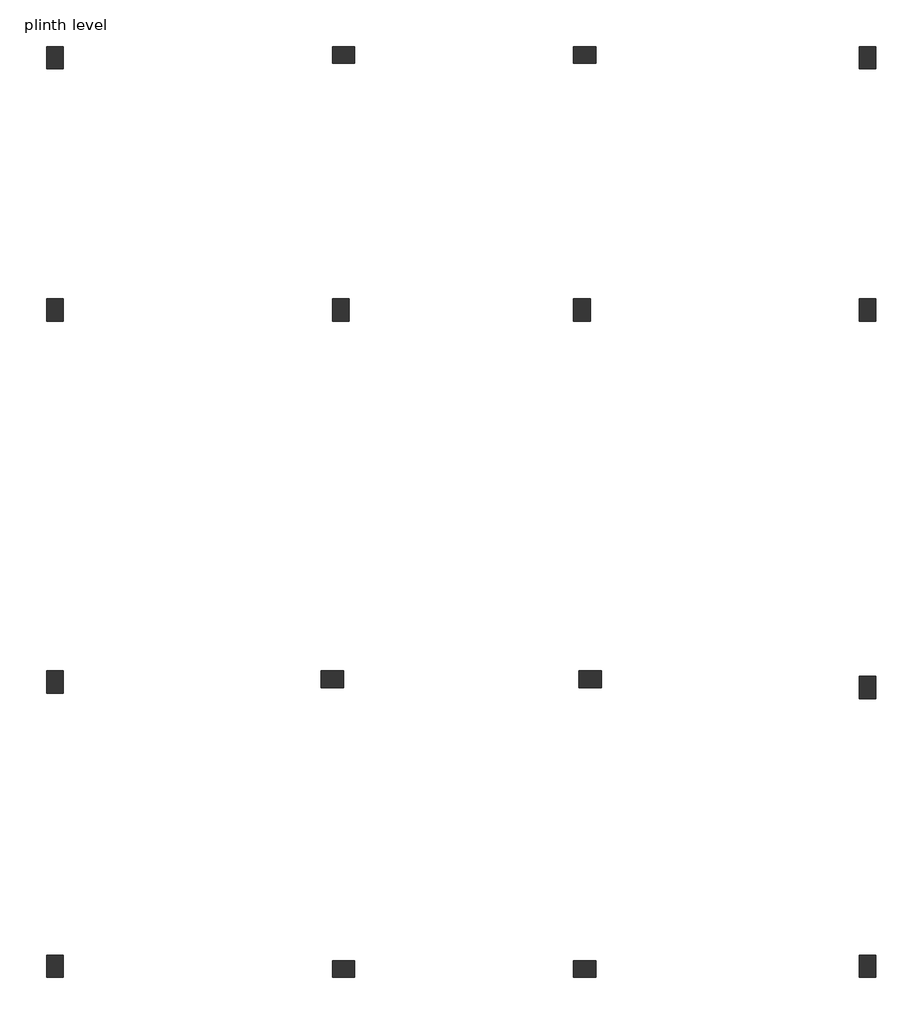
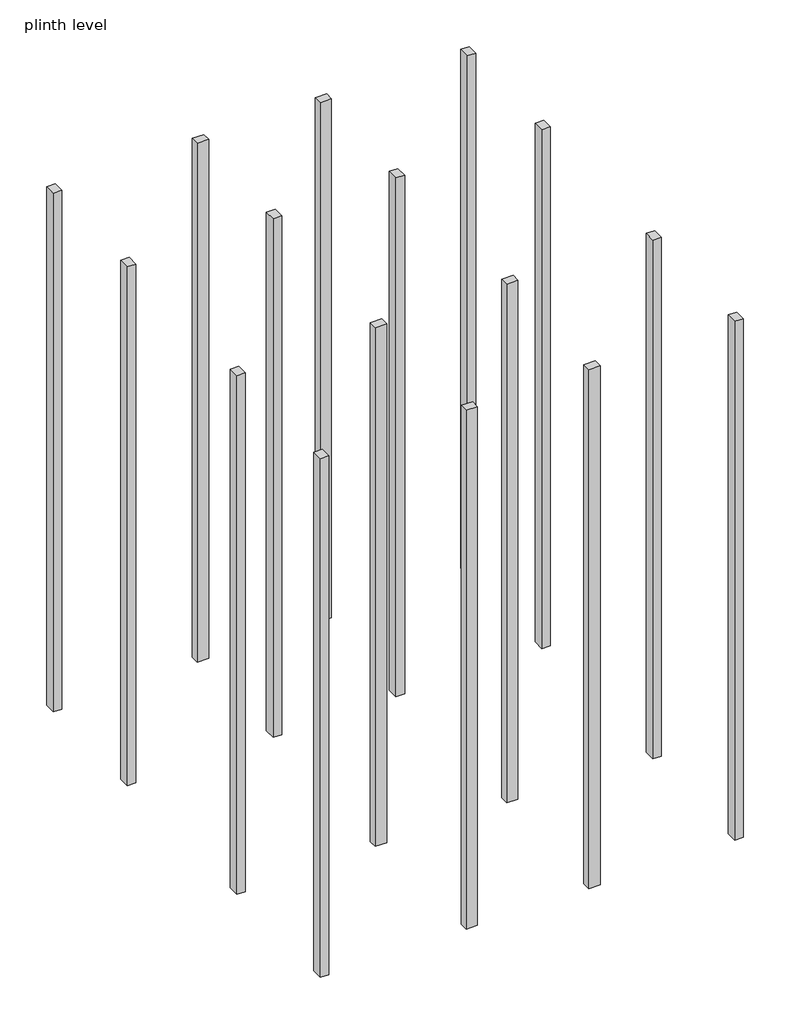
# One storey: 16 columns.
"""IFC4 building model written with IfcOpenShell, lengths in millimetres."""

from ifc_helpers import new_model, si_unit, origin, place, context, project, spatial, faceted_brep, element, save

model = new_model("IFC4")

# Units and contexts
model_context = context("Model", 3, world=origin())
ifc_project = project(units=[si_unit("LENGTHUNIT", "METRE", prefix="MILLI")], contexts=[model_context])

# Site, building, storey
site = spatial("IfcSite", under=ifc_project)
building = spatial("IfcBuilding", under=site)
storey = spatial("IfcBuildingStorey", under=building, Name="plinth level", Elevation=-1219.2)

# Columns
placement = place(None, origin())
element("IfcColumn", 1, ObjectType="Concrete-Rectangular-Column", at=placement, inside=storey, context=model_context, shape_type="Brep", body=[
    faceted_brep([(-12413.6124084, 10180.7961804, -1219.2), (-12413.6124084, 9875.9961804, -1219.2), (-12642.2124084, 9875.9961804, -1219.2), (-12642.2124084, 10180.7961804, -1219.2), (-12413.6124084, 10180.7961804, 13411.2), (-12413.6124084, 9875.9961804, 13411.2), (-12413.6124084, 9875.9961804, 609.6), (-12413.6124084, 9875.9961804, 304.8), (-12642.2124084, 9875.9961804, 13411.2), (-12642.2124084, 9875.9961804, 609.6), (-12642.2124084, 9875.9961804, 304.8), (-12642.2124084, 10180.7961804, 13411.2)], [[[0, 1, 2, 3]], [[4, 5, 6, 7, 1, 0]], [[5, 8, 9, 10, 2, 1, 7, 6]], [[8, 11, 3, 2, 10, 9]], [[11, 4, 0, 3]], [[4, 11, 8, 5]]]),
])
element("IfcColumn", 2, ObjectType="Concrete-Rectangular-Column", at=placement, inside=storey, context=model_context, shape_type="Brep", body=[
    faceted_brep([(-8756.0124084, 10180.7961804, -1219.2), (-8451.2124084, 10180.7961804, -1219.2), (-8451.2124084, 9952.1961804, -1219.2), (-8756.0124084, 9952.1961804, -1219.2), (-8756.0124084, 10180.7961804, 13411.2), (-8451.2124084, 10180.7961804, 13411.2), (-8451.2124084, 9952.1961804, 13411.2), (-8451.2124084, 9952.1961804, 10210.8), (-8451.2124084, 9952.1961804, 9906.0), (-8451.2124084, 9952.1961804, 7010.4), (-8451.2124084, 9952.1961804, 6705.6), (-8451.2124084, 9952.1961804, 3810.0), (-8451.2124084, 9952.1961804, 3505.2), (-8451.2124084, 9952.1961804, 609.6), (-8451.2124084, 9952.1961804, 304.8), (-8756.0124084, 9952.1961804, 13411.2), (-8756.0124084, 9952.1961804, 10210.8), (-8756.0124084, 9952.1961804, 9906.0), (-8756.0124084, 9952.1961804, 7010.4), (-8756.0124084, 9952.1961804, 6705.6), (-8756.0124084, 9952.1961804, 3810.0), (-8756.0124084, 9952.1961804, 3505.2), (-8756.0124084, 9952.1961804, 609.6), (-8756.0124084, 9952.1961804, 304.8)], [[[0, 1, 2, 3]], [[4, 5, 1, 0]], [[5, 6, 7, 8, 9, 10, 11, 12, 13, 14, 2, 1]], [[6, 15, 16, 17, 18, 19, 20, 21, 22, 23, 3, 2, 14, 13, 12, 11, 10, 9, 8, 7]], [[15, 4, 0, 3, 23, 22, 21, 20, 19, 18, 17, 16]], [[4, 15, 6, 5]]]),
])
element("IfcColumn", 3, ObjectType="Concrete-Rectangular-Column", at=placement, inside=storey, context=model_context, shape_type="Brep", body=[
    faceted_brep([(-5479.4124084, 10180.7961804, -1219.2), (-5174.6124084, 10180.7961804, -1219.2), (-5174.6124084, 9952.1961804, -1219.2), (-5479.4124084, 9952.1961804, -1219.2), (-5479.4124084, 10180.7961804, 13411.2), (-5174.6124084, 10180.7961804, 13411.2), (-5174.6124084, 9952.1961804, 13411.2), (-5174.6124084, 9952.1961804, 10210.8), (-5174.6124084, 9952.1961804, 9906.0), (-5174.6124084, 9952.1961804, 7010.4), (-5174.6124084, 9952.1961804, 6705.6), (-5174.6124084, 9952.1961804, 3810.0), (-5174.6124084, 9952.1961804, 3505.2), (-5174.6124084, 9952.1961804, 609.6), (-5174.6124084, 9952.1961804, 304.8), (-5479.4124084, 9952.1961804, 13411.2), (-5479.4124084, 9952.1961804, 10210.8), (-5479.4124084, 9952.1961804, 9906.0), (-5479.4124084, 9952.1961804, 7010.4), (-5479.4124084, 9952.1961804, 6705.6), (-5479.4124084, 9952.1961804, 3810.0), (-5479.4124084, 9952.1961804, 3505.2), (-5479.4124084, 9952.1961804, 609.6), (-5479.4124084, 9952.1961804, 304.8)], [[[0, 1, 2, 3]], [[4, 5, 1, 0]], [[5, 6, 7, 8, 9, 10, 11, 12, 13, 14, 2, 1]], [[6, 15, 16, 17, 18, 19, 20, 21, 22, 23, 3, 2, 14, 13, 12, 11, 10, 9, 8, 7]], [[15, 4, 0, 3, 23, 22, 21, 20, 19, 18, 17, 16]], [[4, 15, 6, 5]]]),
])
element("IfcColumn", 4, ObjectType="Concrete-Rectangular-Column", at=placement, inside=storey, context=model_context, shape_type="Brep", body=[
    faceted_brep([(-1364.6124084, 10180.7961804, -1219.2), (-1364.6124084, 9875.9961804, -1219.2), (-1593.2124084, 9875.9961804, -1219.2), (-1593.2124084, 10180.7961804, -1219.2), (-1364.6124084, 10180.7961804, 13411.2), (-1364.6124084, 9875.9961804, 13411.2), (-1364.6124084, 9875.9961804, 609.6), (-1364.6124084, 9875.9961804, 304.8), (-1593.2124084, 9875.9961804, 13411.2), (-1593.2124084, 9875.9961804, 609.6), (-1593.2124084, 9875.9961804, 304.8), (-1593.2124084, 10180.7961804, 13411.2)], [[[0, 1, 2, 3]], [[4, 5, 6, 7, 1, 0]], [[5, 8, 9, 10, 2, 1, 7, 6]], [[8, 11, 3, 2, 10, 9]], [[11, 4, 0, 3]], [[4, 11, 8, 5]]]),
])
element("IfcColumn", 5, ObjectType="Concrete-Rectangular-Column", at=placement, inside=storey, context=model_context, shape_type="Brep", body=[
    faceted_brep([(-1364.6124084, 6751.7961804, -1219.2), (-1364.6124084, 6446.9961804, -1219.2), (-1593.2124084, 6446.9961804, -1219.2), (-1593.2124084, 6751.7961804, -1219.2), (-1364.6124084, 6751.7961804, 13411.2), (-1364.6124084, 6446.9961804, 13411.2), (-1364.6124084, 6751.7961804, 304.8), (-1364.6124084, 6751.7961804, 609.6), (-1593.2124084, 6446.9961804, 13411.2), (-1593.2124084, 6751.7961804, 13411.2), (-1593.2124084, 6751.7961804, 609.6), (-1593.2124084, 6751.7961804, 304.8)], [[[0, 1, 2, 3]], [[4, 5, 1, 0, 6, 7]], [[5, 8, 2, 1]], [[8, 9, 10, 11, 3, 2]], [[9, 4, 7, 6, 0, 3, 11, 10]], [[4, 9, 8, 5]]]),
])
element("IfcColumn", 6, ObjectType="Concrete-Rectangular-Column", at=placement, inside=storey, context=model_context, shape_type="Brep", body=[
    faceted_brep([(-1364.6124084, 1620.9961804, -1219.2), (-1364.6124084, 1316.1961804, -1219.2), (-1593.2124084, 1316.1961804, -1219.2), (-1593.2124084, 1620.9961804, -1219.2), (-1364.6124084, 1620.9961804, 13411.2), (-1364.6124084, 1316.1961804, 13411.2), (-1364.6124084, 1316.1961804, 609.6), (-1364.6124084, 1316.1961804, 304.8), (-1364.6124084, 1620.9961804, 304.8), (-1364.6124084, 1620.9961804, 609.6), (-1364.6124084, 1620.9961804, 3505.2), (-1364.6124084, 1620.9961804, 3810.0), (-1364.6124084, 1620.9961804, 6705.6), (-1364.6124084, 1620.9961804, 7010.4), (-1364.6124084, 1620.9961804, 9906.0), (-1364.6124084, 1620.9961804, 10210.8), (-1593.2124084, 1316.1961804, 13411.2), (-1593.2124084, 1316.1961804, 609.6), (-1593.2124084, 1316.1961804, 304.8), (-1593.2124084, 1620.9961804, 13411.2), (-1593.2124084, 1620.9961804, 10210.8), (-1593.2124084, 1620.9961804, 9906.0), (-1593.2124084, 1620.9961804, 7010.4), (-1593.2124084, 1620.9961804, 6705.6), (-1593.2124084, 1620.9961804, 3810.0), (-1593.2124084, 1620.9961804, 3505.2), (-1593.2124084, 1620.9961804, 609.6), (-1593.2124084, 1620.9961804, 304.8)], [[[0, 1, 2, 3]], [[4, 5, 6, 7, 1, 0, 8, 9, 10, 11, 12, 13, 14, 15]], [[5, 16, 17, 18, 2, 1, 7, 6]], [[16, 19, 20, 21, 22, 23, 24, 25, 26, 27, 3, 2, 18, 17]], [[19, 4, 15, 14, 13, 12, 11, 10, 9, 8, 0, 3, 27, 26, 25, 24, 23, 22, 21, 20]], [[4, 19, 16, 5]]]),
])
element("IfcColumn", 7, ObjectType="Concrete-Rectangular-Column", at=placement, inside=storey, context=model_context, shape_type="Brep", body=[
    faceted_brep([(-1364.6124084, -2163.6038196, -1219.2), (-1364.6124084, -2468.4038196, -1219.2), (-1593.2124084, -2468.4038196, -1219.2), (-1593.2124084, -2163.6038196, -1219.2), (-1364.6124084, -2163.6038196, 13411.2), (-1364.6124084, -2468.4038196, 13411.2), (-1364.6124084, -2163.6038196, 304.8), (-1364.6124084, -2163.6038196, 609.6), (-1593.2124084, -2468.4038196, 13411.2), (-1593.2124084, -2163.6038196, 13411.2), (-1593.2124084, -2163.6038196, 609.6), (-1593.2124084, -2163.6038196, 304.8)], [[[0, 1, 2, 3]], [[4, 5, 1, 0, 6, 7]], [[5, 8, 2, 1]], [[8, 9, 10, 11, 3, 2]], [[9, 4, 7, 6, 0, 3, 11, 10]], [[4, 9, 8, 5]]]),
])
element("IfcColumn", 8, ObjectType="Concrete-Rectangular-Column", at=placement, inside=storey, context=model_context, shape_type="Brep", body=[
    faceted_brep([(-5479.4124084, -2239.8038196, -1219.2), (-5174.6124084, -2239.8038196, -1219.2), (-5174.6124084, -2468.4038196, -1219.2), (-5479.4124084, -2468.4038196, -1219.2), (-5479.4124084, -2239.8038196, 13411.2), (-5174.6124084, -2239.8038196, 13411.2), (-5174.6124084, -2239.8038196, 609.6), (-5174.6124084, -2239.8038196, 304.8), (-5174.6124084, -2468.4038196, 13411.2), (-5479.4124084, -2468.4038196, 13411.2)], [[[0, 1, 2, 3]], [[4, 5, 6, 7, 1, 0]], [[5, 8, 2, 1, 7, 6]], [[8, 9, 3, 2]], [[9, 4, 0, 3]], [[4, 9, 8, 5]]]),
])
element("IfcColumn", 9, ObjectType="Concrete-Rectangular-Column", at=placement, inside=storey, context=model_context, shape_type="Brep", body=[
    faceted_brep([(-8756.0124084, -2239.8038196, -1219.2), (-8451.2124084, -2239.8038196, -1219.2), (-8451.2124084, -2468.4038196, -1219.2), (-8756.0124084, -2468.4038196, -1219.2), (-8756.0124084, -2239.8038196, 13411.2), (-8451.2124084, -2239.8038196, 13411.2), (-8756.0124084, -2239.8038196, 304.8), (-8756.0124084, -2239.8038196, 609.6), (-8451.2124084, -2468.4038196, 13411.2), (-8756.0124084, -2468.4038196, 13411.2), (-8756.0124084, -2468.4038196, 609.6), (-8756.0124084, -2468.4038196, 304.8)], [[[0, 1, 2, 3]], [[4, 5, 1, 0, 6, 7]], [[5, 8, 2, 1]], [[8, 9, 10, 11, 3, 2]], [[9, 4, 7, 6, 0, 3, 11, 10]], [[4, 9, 8, 5]]]),
])
element("IfcColumn", 10, ObjectType="Concrete-Rectangular-Column", at=placement, inside=storey, context=model_context, shape_type="Brep", body=[
    faceted_brep([(-12642.2124084, -2468.4038196, -1219.2), (-12642.2124084, -2163.6038196, -1219.2), (-12413.6124084, -2163.6038196, -1219.2), (-12413.6124084, -2468.4038196, -1219.2), (-12642.2124084, -2468.4038196, 13411.2), (-12642.2124084, -2163.6038196, 13411.2), (-12642.2124084, -2163.6038196, 609.6), (-12642.2124084, -2163.6038196, 304.8), (-12413.6124084, -2163.6038196, 13411.2), (-12413.6124084, -2163.6038196, 609.6), (-12413.6124084, -2163.6038196, 304.8), (-12413.6124084, -2468.4038196, 13411.2), (-12413.6124084, -2468.4038196, 609.6), (-12413.6124084, -2468.4038196, 304.8)], [[[0, 1, 2, 3]], [[4, 5, 6, 7, 1, 0]], [[5, 8, 9, 10, 2, 1, 7, 6]], [[8, 11, 12, 13, 3, 2, 10, 9]], [[11, 4, 0, 3, 13, 12]], [[4, 11, 8, 5]]]),
])
element("IfcColumn", 11, ObjectType="Concrete-Rectangular-Column", at=placement, inside=storey, context=model_context, shape_type="Brep", body=[
    faceted_brep([(-12413.6124084, 1697.1961804, -1219.2), (-12413.6124084, 1392.3961804, -1219.2), (-12642.2124084, 1392.3961804, -1219.2), (-12642.2124084, 1697.1961804, -1219.2), (-12413.6124084, 1697.1961804, 13411.2), (-12413.6124084, 1392.3961804, 13411.2), (-12413.6124084, 1392.3961804, 10210.8), (-12413.6124084, 1392.3961804, 9906.0), (-12413.6124084, 1392.3961804, 7010.4), (-12413.6124084, 1392.3961804, 6705.6), (-12413.6124084, 1392.3961804, 3810.0), (-12413.6124084, 1392.3961804, 3505.2), (-12413.6124084, 1392.3961804, 609.6), (-12413.6124084, 1392.3961804, 304.8), (-12413.6124084, 1697.1961804, 304.8), (-12413.6124084, 1697.1961804, 609.6), (-12413.6124084, 1697.1961804, 3505.2), (-12413.6124084, 1697.1961804, 3810.0), (-12413.6124084, 1697.1961804, 6705.6), (-12413.6124084, 1697.1961804, 7010.4), (-12413.6124084, 1697.1961804, 9906.0), (-12413.6124084, 1697.1961804, 10210.8), (-12642.2124084, 1392.3961804, 13411.2), (-12642.2124084, 1392.3961804, 10210.8), (-12642.2124084, 1392.3961804, 9906.0), (-12642.2124084, 1392.3961804, 7010.4), (-12642.2124084, 1392.3961804, 6705.6), (-12642.2124084, 1392.3961804, 3810.0), (-12642.2124084, 1392.3961804, 3505.2), (-12642.2124084, 1392.3961804, 609.6), (-12642.2124084, 1392.3961804, 304.8), (-12642.2124084, 1697.1961804, 13411.2), (-12642.2124084, 1697.1961804, 10210.8), (-12642.2124084, 1697.1961804, 9906.0), (-12642.2124084, 1697.1961804, 7010.4), (-12642.2124084, 1697.1961804, 6705.6), (-12642.2124084, 1697.1961804, 3810.0), (-12642.2124084, 1697.1961804, 3505.2), (-12642.2124084, 1697.1961804, 609.6), (-12642.2124084, 1697.1961804, 304.8)], [[[0, 1, 2, 3]], [[4, 5, 6, 7, 8, 9, 10, 11, 12, 13, 1, 0, 14, 15, 16, 17, 18, 19, 20, 21]], [[5, 22, 23, 24, 25, 26, 27, 28, 29, 30, 2, 1, 13, 12, 11, 10, 9, 8, 7, 6]], [[22, 31, 32, 33, 34, 35, 36, 37, 38, 39, 3, 2, 30, 29, 28, 27, 26, 25, 24, 23]], [[31, 4, 21, 20, 19, 18, 17, 16, 15, 14, 0, 3, 39, 38, 37, 36, 35, 34, 33, 32]], [[4, 31, 22, 5]]]),
])
element("IfcColumn", 12, ObjectType="Concrete-Rectangular-Column", at=placement, inside=storey, context=model_context, shape_type="Brep", body=[
    faceted_brep([(-12413.6124084, 6751.7961804, -1219.2), (-12413.6124084, 6446.9961804, -1219.2), (-12642.2124084, 6446.9961804, -1219.2), (-12642.2124084, 6751.7961804, -1219.2), (-12413.6124084, 6751.7961804, 13411.2), (-12413.6124084, 6446.9961804, 13411.2), (-12413.6124084, 6446.9961804, 10210.8), (-12413.6124084, 6446.9961804, 9906.0), (-12413.6124084, 6446.9961804, 7010.4), (-12413.6124084, 6446.9961804, 6705.6), (-12413.6124084, 6446.9961804, 3810.0), (-12413.6124084, 6446.9961804, 3505.2), (-12413.6124084, 6446.9961804, 609.6), (-12413.6124084, 6446.9961804, 304.8), (-12413.6124084, 6751.7961804, 304.8), (-12413.6124084, 6751.7961804, 609.6), (-12413.6124084, 6751.7961804, 3505.2), (-12413.6124084, 6751.7961804, 3810.0), (-12413.6124084, 6751.7961804, 6705.6), (-12413.6124084, 6751.7961804, 7010.4), (-12413.6124084, 6751.7961804, 9906.0), (-12413.6124084, 6751.7961804, 10210.8), (-12642.2124084, 6446.9961804, 13411.2), (-12642.2124084, 6446.9961804, 10210.8), (-12642.2124084, 6446.9961804, 9906.0), (-12642.2124084, 6446.9961804, 7010.4), (-12642.2124084, 6446.9961804, 6705.6), (-12642.2124084, 6446.9961804, 3810.0), (-12642.2124084, 6446.9961804, 3505.2), (-12642.2124084, 6446.9961804, 609.6), (-12642.2124084, 6446.9961804, 304.8), (-12642.2124084, 6751.7961804, 13411.2), (-12642.2124084, 6751.7961804, 10210.8), (-12642.2124084, 6751.7961804, 9906.0), (-12642.2124084, 6751.7961804, 7010.4), (-12642.2124084, 6751.7961804, 6705.6), (-12642.2124084, 6751.7961804, 3810.0), (-12642.2124084, 6751.7961804, 3505.2), (-12642.2124084, 6751.7961804, 609.6), (-12642.2124084, 6751.7961804, 304.8)], [[[0, 1, 2, 3]], [[4, 5, 6, 7, 8, 9, 10, 11, 12, 13, 1, 0, 14, 15, 16, 17, 18, 19, 20, 21]], [[5, 22, 23, 24, 25, 26, 27, 28, 29, 30, 2, 1, 13, 12, 11, 10, 9, 8, 7, 6]], [[22, 31, 32, 33, 34, 35, 36, 37, 38, 39, 3, 2, 30, 29, 28, 27, 26, 25, 24, 23]], [[31, 4, 21, 20, 19, 18, 17, 16, 15, 14, 0, 3, 39, 38, 37, 36, 35, 34, 33, 32]], [[4, 31, 22, 5]]]),
])
element("IfcColumn", 13, ObjectType="Concrete-Rectangular-Column", at=placement, inside=storey, context=model_context, shape_type="Brep", body=[
    faceted_brep([(-8527.4124084, 6751.7961804, -1219.2), (-8527.4124084, 6446.9961804, -1219.2), (-8756.0124084, 6446.9961804, -1219.2), (-8756.0124084, 6751.7961804, -1219.2), (-8527.4124084, 6751.7961804, 13411.2), (-8527.4124084, 6446.9961804, 13411.2), (-8756.0124084, 6446.9961804, 13411.2), (-8756.0124084, 6446.9961804, 10210.8), (-8756.0124084, 6446.9961804, 9906.0), (-8756.0124084, 6446.9961804, 7010.4), (-8756.0124084, 6446.9961804, 6705.6), (-8756.0124084, 6446.9961804, 3810.0), (-8756.0124084, 6446.9961804, 3505.2), (-8756.0124084, 6446.9961804, 609.6), (-8756.0124084, 6446.9961804, 304.8), (-8756.0124084, 6751.7961804, 13411.2), (-8756.0124084, 6751.7961804, 10210.8), (-8756.0124084, 6751.7961804, 9906.0), (-8756.0124084, 6751.7961804, 7010.4), (-8756.0124084, 6751.7961804, 6705.6), (-8756.0124084, 6751.7961804, 3810.0), (-8756.0124084, 6751.7961804, 3505.2), (-8756.0124084, 6751.7961804, 609.6), (-8756.0124084, 6751.7961804, 304.8)], [[[0, 1, 2, 3]], [[4, 5, 1, 0]], [[5, 6, 7, 8, 9, 10, 11, 12, 13, 14, 2, 1]], [[6, 15, 16, 17, 18, 19, 20, 21, 22, 23, 3, 2, 14, 13, 12, 11, 10, 9, 8, 7]], [[15, 4, 0, 3, 23, 22, 21, 20, 19, 18, 17, 16]], [[4, 15, 6, 5]]]),
])
element("IfcColumn", 14, ObjectType="Concrete-Rectangular-Column", at=placement, inside=storey, context=model_context, shape_type="Brep", body=[
    faceted_brep([(-5250.8124084, 6751.7961804, -1219.2), (-5250.8124084, 6446.9961804, -1219.2), (-5479.4124084, 6446.9961804, -1219.2), (-5479.4124084, 6751.7961804, -1219.2), (-5250.8124084, 6751.7961804, 13411.2), (-5250.8124084, 6446.9961804, 13411.2), (-5250.8124084, 6446.9961804, 10210.8), (-5250.8124084, 6446.9961804, 9906.0), (-5250.8124084, 6446.9961804, 7010.4), (-5250.8124084, 6446.9961804, 6705.6), (-5250.8124084, 6446.9961804, 3810.0), (-5250.8124084, 6446.9961804, 3505.2), (-5250.8124084, 6446.9961804, 609.6), (-5250.8124084, 6446.9961804, 304.8), (-5250.8124084, 6751.7961804, 304.8), (-5250.8124084, 6751.7961804, 609.6), (-5250.8124084, 6751.7961804, 3505.2), (-5250.8124084, 6751.7961804, 3810.0), (-5250.8124084, 6751.7961804, 6705.6), (-5250.8124084, 6751.7961804, 7010.4), (-5250.8124084, 6751.7961804, 9906.0), (-5250.8124084, 6751.7961804, 10210.8), (-5479.4124084, 6446.9961804, 13411.2), (-5479.4124084, 6751.7961804, 13411.2)], [[[0, 1, 2, 3]], [[4, 5, 6, 7, 8, 9, 10, 11, 12, 13, 1, 0, 14, 15, 16, 17, 18, 19, 20, 21]], [[5, 22, 2, 1, 13, 12, 11, 10, 9, 8, 7, 6]], [[22, 23, 3, 2]], [[23, 4, 21, 20, 19, 18, 17, 16, 15, 14, 0, 3]], [[4, 23, 22, 5]]]),
])
element("IfcColumn", 15, ObjectType="Concrete-Rectangular-Column", at=placement, inside=storey, context=model_context, shape_type="Brep", body=[
    faceted_brep([(-8908.4124084, 1697.1961804, -1219.2), (-8603.6124084, 1697.1961804, -1219.2), (-8603.6124084, 1468.5961804, -1219.2), (-8908.4124084, 1468.5961804, -1219.2), (-8908.4124084, 1697.1961804, 13411.2), (-8603.6124084, 1697.1961804, 13411.2), (-8603.6124084, 1697.1961804, 10210.8), (-8603.6124084, 1697.1961804, 9906.0), (-8603.6124084, 1697.1961804, 7010.4), (-8603.6124084, 1697.1961804, 6705.6), (-8603.6124084, 1697.1961804, 3810.0), (-8603.6124084, 1697.1961804, 3505.2), (-8603.6124084, 1697.1961804, 609.6), (-8603.6124084, 1697.1961804, 304.8), (-8603.6124084, 1468.5961804, 13411.2), (-8603.6124084, 1468.5961804, 10210.8), (-8603.6124084, 1468.5961804, 9906.0), (-8603.6124084, 1468.5961804, 7010.4), (-8603.6124084, 1468.5961804, 6705.6), (-8603.6124084, 1468.5961804, 3810.0), (-8603.6124084, 1468.5961804, 3505.2), (-8603.6124084, 1468.5961804, 609.6), (-8603.6124084, 1468.5961804, 304.8), (-8908.4124084, 1468.5961804, 13411.2), (-8908.4124084, 1468.5961804, 10210.8), (-8908.4124084, 1468.5961804, 9906.0), (-8908.4124084, 1468.5961804, 7010.4), (-8908.4124084, 1468.5961804, 6705.6), (-8908.4124084, 1468.5961804, 3810.0), (-8908.4124084, 1468.5961804, 3505.2), (-8908.4124084, 1468.5961804, 609.6), (-8908.4124084, 1468.5961804, 304.8)], [[[0, 1, 2, 3]], [[4, 5, 6, 7, 8, 9, 10, 11, 12, 13, 1, 0]], [[5, 14, 15, 16, 17, 18, 19, 20, 21, 22, 2, 1, 13, 12, 11, 10, 9, 8, 7, 6]], [[14, 23, 24, 25, 26, 27, 28, 29, 30, 31, 3, 2, 22, 21, 20, 19, 18, 17, 16, 15]], [[23, 4, 0, 3, 31, 30, 29, 28, 27, 26, 25, 24]], [[4, 23, 14, 5]]]),
])
element("IfcColumn", 16, ObjectType="Concrete-Rectangular-Column", at=placement, inside=storey, context=model_context, shape_type="Brep", body=[
    faceted_brep([(-5403.2124084, 1697.1961804, -1219.2), (-5098.4124084, 1697.1961804, -1219.2), (-5098.4124084, 1468.5961804, -1219.2), (-5403.2124084, 1468.5961804, -1219.2), (-5403.2124084, 1697.1961804, 13411.2), (-5098.4124084, 1697.1961804, 13411.2), (-5403.2124084, 1697.1961804, 304.8), (-5403.2124084, 1697.1961804, 609.6), (-5403.2124084, 1697.1961804, 3505.2), (-5403.2124084, 1697.1961804, 3810.0), (-5403.2124084, 1697.1961804, 6705.6), (-5403.2124084, 1697.1961804, 7010.4), (-5403.2124084, 1697.1961804, 9906.0), (-5403.2124084, 1697.1961804, 10210.8), (-5098.4124084, 1468.5961804, 13411.2), (-5098.4124084, 1468.5961804, 10210.8), (-5098.4124084, 1468.5961804, 9906.0), (-5098.4124084, 1468.5961804, 7010.4), (-5098.4124084, 1468.5961804, 6705.6), (-5098.4124084, 1468.5961804, 3810.0), (-5098.4124084, 1468.5961804, 3505.2), (-5098.4124084, 1468.5961804, 609.6), (-5098.4124084, 1468.5961804, 304.8), (-5403.2124084, 1468.5961804, 13411.2), (-5403.2124084, 1468.5961804, 10210.8), (-5403.2124084, 1468.5961804, 9906.0), (-5403.2124084, 1468.5961804, 7010.4), (-5403.2124084, 1468.5961804, 6705.6), (-5403.2124084, 1468.5961804, 3810.0), (-5403.2124084, 1468.5961804, 3505.2), (-5403.2124084, 1468.5961804, 609.6), (-5403.2124084, 1468.5961804, 304.8)], [[[0, 1, 2, 3]], [[4, 5, 1, 0, 6, 7, 8, 9, 10, 11, 12, 13]], [[5, 14, 15, 16, 17, 18, 19, 20, 21, 22, 2, 1]], [[14, 23, 24, 25, 26, 27, 28, 29, 30, 31, 3, 2, 22, 21, 20, 19, 18, 17, 16, 15]], [[23, 4, 13, 12, 11, 10, 9, 8, 7, 6, 0, 3, 31, 30, 29, 28, 27, 26, 25, 24]], [[4, 23, 14, 5]]]),
])

save(model, "model.ifc")

# Revit data of these elements
# Type "Concrete-Rectangular-Column"
#   Assembly Code = "B10"
#   b = 0' - 9"
#   h = 1' - 0"
#   Structural Material [instance default] = Concrete, Cast-in-Place gray
# Elements 1, 2, 3, 4, 5, 6, 7, 8, 9, 10, 11, 12, 13, 14, 15, 16 (IfcColumn, "Concrete-Rectangular-Column")
#   Structural Material = Concrete, Cast-in-Place gray
#   Phase Created = New Construction
#   Materials on its faces: "Concrete, Cast-in-Place gray"
# Materials
#   "Concrete, Cast-in-Place gray": class "Concrete", colour RGB 192 192 192, transparency 0, Description = "Cast-in-place concrete", Cost = 0
